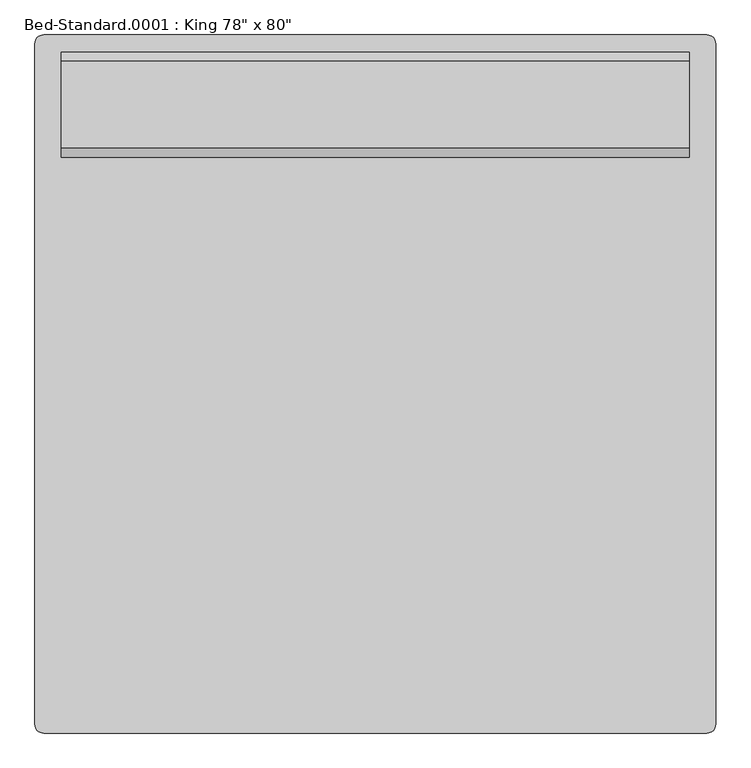
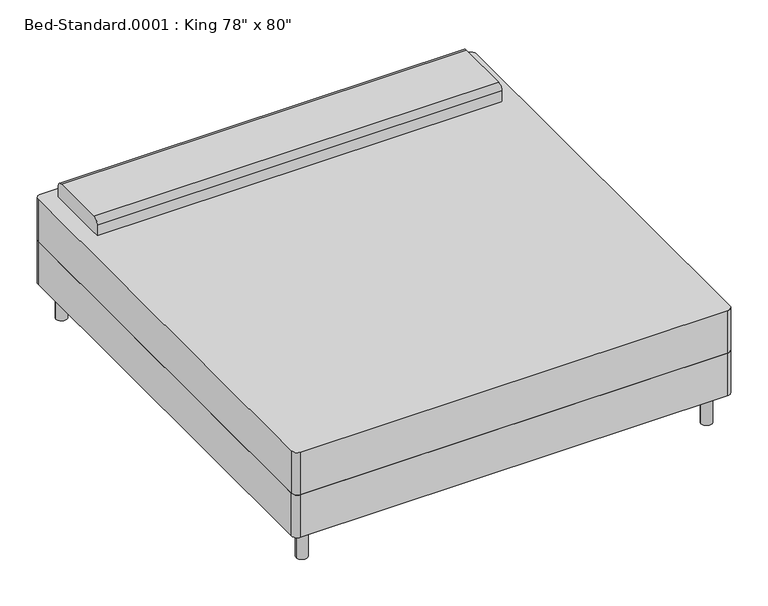
"""IFC4 building model written with IfcOpenShell, lengths in millimetres: furniture geometry."""

from ifc_helpers import new_model, si_unit, point, frame, frame_2d, origin, origin_with_axes, place, context, project, spatial, polyline, circle_curve, trimmed, segment, composite_curve, outline, extrude, source, transform, mapped, element, save


def furniture_1fc5af50(model_context):
    return source(origin(), model_context, "Body", "SweptSolid", [
        extrude(outline(composite_curve([segment(polyline([(-719.1114754, -1036.195082), (-719.1114754, 945.004918)]), True, "CONTINUOUS"), segment(trimmed(circle_curve(frame_2d((-693.7114754, 945.004918)), 25.4), [point((-719.1114754, 945.004918))], [point((-693.7114754, 970.404918))], False, "CARTESIAN"), True, "CONTINUOUS"), segment(polyline([(-693.7114754, 970.404918), (1236.6885246, 970.404918)]), True, "CONTINUOUS"), segment(trimmed(circle_curve(frame_2d((1236.6885246, 945.004918)), 25.4), [point((1236.6885246, 970.404918))], [point((1262.0885246, 945.004918))], False, "CARTESIAN"), True, "CONTINUOUS"), segment(polyline([(1262.0885246, 945.004918), (1262.0885246, -1036.195082)]), True, "CONTINUOUS"), segment(trimmed(circle_curve(frame_2d((1236.6885246, -1036.195082)), 25.4), [point((1262.0885246, -1036.195082))], [point((1236.6885246, -1061.595082))], False, "CARTESIAN"), True, "CONTINUOUS"), segment(polyline([(1236.6885246, -1061.595082), (-693.7114754, -1061.595082)]), True, "CONTINUOUS"), segment(trimmed(circle_curve(frame_2d((-693.7114754, -1036.195082)), 25.4), [point((-693.7114754, -1061.595082))], [point((-719.1114754, -1036.195082))], False, "CARTESIAN"), True, "CONTINUOUS")], self_intersect=False)), frame((0.0, 0.0, 152.4), z_axis=(0.0, 0.0, 1.0), x_axis=(1.0, 0.0, 0.0)), (0.0, 0.0, 1.0), 203.2),
        extrude(outline(composite_curve([segment(polyline([(614.804918, 558.8), (614.804918, 609.6)]), True, "CONTINUOUS"), segment(trimmed(circle_curve(frame_2d((640.204918, 609.6)), 25.4), [point((614.804918, 609.6))], [point((640.204918, 635.0))], False, "CARTESIAN"), True, "CONTINUOUS"), segment(polyline([(640.204918, 635.0), (894.204918, 635.0)]), True, "CONTINUOUS"), segment(trimmed(circle_curve(frame_2d((894.204918, 609.6)), 25.4), [point((894.204918, 635.0))], [point((919.604918, 609.6))], False, "CARTESIAN"), True, "CONTINUOUS"), segment(polyline([(919.604918, 609.6), (919.604918, 558.8), (614.804918, 558.8)]), True, "CONTINUOUS")], self_intersect=False)), frame((-642.9114754, 0.0, 0.0), z_axis=(1.0, 0.0, 0.0), x_axis=(0.0, 1.0, 0.0)), (0.0, 0.0, 1.0), 1828.8),
        extrude(outline(composite_curve([segment(trimmed(circle_curve(frame_2d((-642.9114754, 894.204918)), 25.4), [point((-668.3114754, 894.204918))], [point((-617.5114754, 894.204918))], False, "CARTESIAN"), True, "CONTINUOUS"), segment(trimmed(circle_curve(frame_2d((-642.9114754, 894.204918)), 25.4), [point((-617.5114754, 894.204918))], [point((-668.3114754, 894.204918))], False, "CARTESIAN"), True, "CONTINUOUS")], self_intersect=False)), origin_with_axes(), (0.0, 0.0, 1.0), 152.4),
        extrude(outline(composite_curve([segment(trimmed(circle_curve(frame_2d((1185.8885246, 894.204918)), 25.4), [point((1160.4885246, 894.204918))], [point((1211.2885246, 894.204918))], False, "CARTESIAN"), True, "CONTINUOUS"), segment(trimmed(circle_curve(frame_2d((1185.8885246, 894.204918)), 25.4), [point((1211.2885246, 894.204918))], [point((1160.4885246, 894.204918))], False, "CARTESIAN"), True, "CONTINUOUS")], self_intersect=False)), origin_with_axes(), (0.0, 0.0, 1.0), 152.4),
        extrude(outline(composite_curve([segment(trimmed(circle_curve(frame_2d((1185.8885246, -985.395082)), 25.4), [point((1160.4885246, -985.395082))], [point((1211.2885246, -985.395082))], False, "CARTESIAN"), True, "CONTINUOUS"), segment(trimmed(circle_curve(frame_2d((1185.8885246, -985.395082)), 25.4), [point((1211.2885246, -985.395082))], [point((1160.4885246, -985.395082))], False, "CARTESIAN"), True, "CONTINUOUS")], self_intersect=False)), origin_with_axes(), (0.0, 0.0, 1.0), 152.4),
        extrude(outline(composite_curve([segment(trimmed(circle_curve(frame_2d((-642.9114754, -985.395082)), 25.4), [point((-668.3114754, -985.395082))], [point((-617.5114754, -985.395082))], False, "CARTESIAN"), True, "CONTINUOUS"), segment(trimmed(circle_curve(frame_2d((-642.9114754, -985.395082)), 25.4), [point((-617.5114754, -985.395082))], [point((-668.3114754, -985.395082))], False, "CARTESIAN"), True, "CONTINUOUS")], self_intersect=False)), origin_with_axes(), (0.0, 0.0, 1.0), 152.4),
        extrude(outline(composite_curve([segment(polyline([(-693.7114754, 970.404918), (1236.6885246, 970.404918)]), True, "CONTINUOUS"), segment(trimmed(circle_curve(frame_2d((1236.6885246, 945.004918)), 25.4), [point((1236.6885246, 970.404918))], [point((1262.0885246, 945.004918))], False, "CARTESIAN"), True, "CONTINUOUS"), segment(polyline([(1262.0885246, 945.004918), (1262.0885246, -1036.195082)]), True, "CONTINUOUS"), segment(trimmed(circle_curve(frame_2d((1236.6885246, -1036.195082)), 25.4), [point((1262.0885246, -1036.195082))], [point((1236.6885246, -1061.595082))], False, "CARTESIAN"), True, "CONTINUOUS"), segment(polyline([(1236.6885246, -1061.595082), (-693.7114754, -1061.595082)]), True, "CONTINUOUS"), segment(trimmed(circle_curve(frame_2d((-693.7114754, -1036.195082)), 25.4), [point((-693.7114754, -1061.595082))], [point((-719.1114754, -1036.195082))], False, "CARTESIAN"), True, "CONTINUOUS"), segment(polyline([(-719.1114754, -1036.195082), (-719.1114754, 945.004918)]), True, "CONTINUOUS"), segment(trimmed(circle_curve(frame_2d((-693.7114754, 945.004918)), 25.4), [point((-719.1114754, 945.004918))], [point((-693.7114754, 970.404918))], False, "CARTESIAN"), True, "CONTINUOUS")], self_intersect=False)), frame((0.0, 0.0, 355.6), z_axis=(0.0, 0.0, 1.0), x_axis=(1.0, 0.0, 0.0)), (0.0, 0.0, 1.0), 203.2),
    ])


if __name__ == "__main__":
    model = new_model("IFC4")
    model_context = context("Model", 3, world=origin())
    ifc_project = project(units=[si_unit("LENGTHUNIT", "METRE", prefix="MILLI")], contexts=[model_context])
    site = spatial("IfcSite", under=ifc_project)
    building = spatial("IfcBuilding", under=site)
    placement = place(None, origin())
    furniture_shape = furniture_1fc5af50(model_context)
    element("IfcFurniture", 1, ObjectType="Bed-Standard.0001 : King 78\" x 80\"", at=placement, inside=building, context=model_context, shape_type="MappedRepresentation", body=[
        mapped(furniture_shape, transform((0.0, 0.0, 0.0), x_axis=(1.0, 0.0, 0.0), y_axis=(0.0, 1.0, 0.0), z_axis=(0.0, 0.0, 1.0))),
    ])
    save(model, "model.ifc")

# Revit data of these elements
# Type "Bed-Standard.0001 : King 78\" x 80\""
#   Assembly Code = "E2020200"
#   Length = 6' - 8"
#   Width = 6' - 6"
#   Leg Material = Steel, Chrome Plated
#   Mattress Material = Linen, White
#   Default Elevation = 0
# Element 1 (IfcFurniture, "Bed-Standard.0001 : King 78\" x 80\"")
#   Materials on its faces: "Linen, White", "Steel, Chrome Plated"
# Materials
#   "Steel, Chrome Plated": class "Metal", colour RGB 17 17 17, transparency 0, Description = "Chromiuim plated steel", Cost = 0
#   "Linen, White": class "Textile", colour RGB 247 247 239, transparency 0, Description = "Linen, white", Cost = 0
